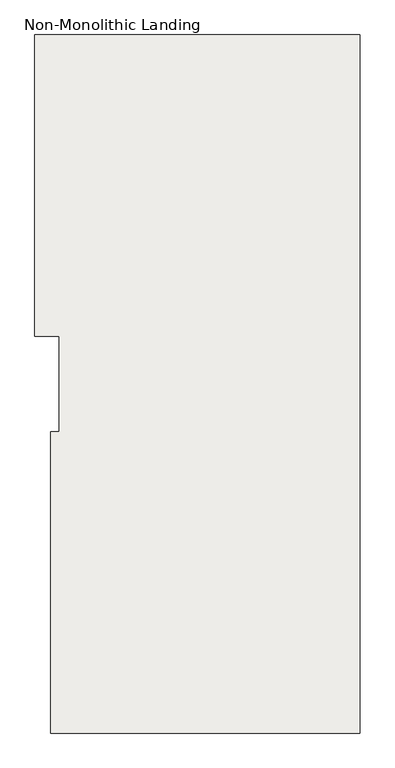
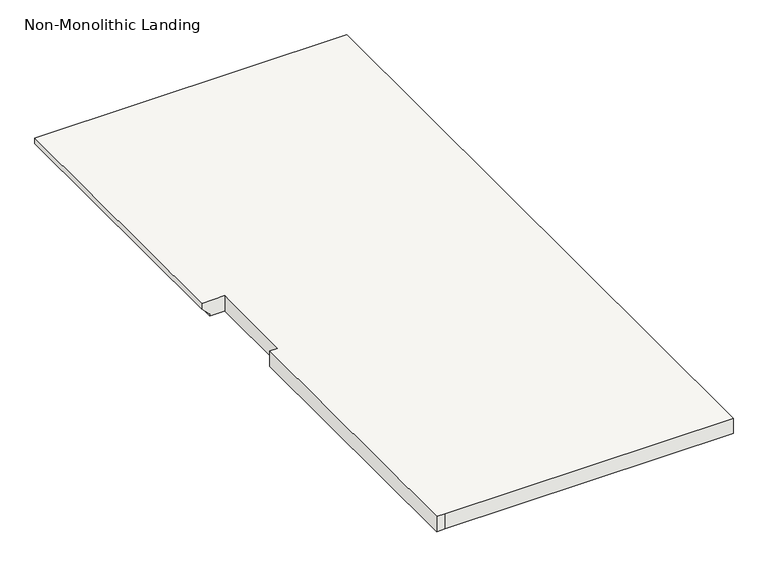
"""IFC4 building model written with IfcOpenShell, lengths in millimetres: slab geometry, Non-Monolithic Landing."""

from ifc_helpers import new_model, si_unit, origin, place, context, project, spatial, faceted_brep, source, transform, mapped, element, save


def non_monolithic_landing_a5fdca2b(model_context):
    return source(origin(), model_context, "Body", "Brep", [
        faceted_brep([(-6915.3703437, -6347.7504041, 4891.6166667), (-6915.3703437, -6347.7504041, 4910.6666667), (-6915.3703437, -5433.3504041, 4910.6666667), (-6915.3703437, -5433.3504041, 4891.6166667), (-6889.9703437, -6347.7504041, 4866.2166667), (-6889.9703437, -5433.3504041, 4866.2166667), (-6841.3260609, -6347.7504041, 4910.6666667), (-6841.3260609, -6639.0810793, 4910.6666667), (-6866.7260609, -6639.0810793, 4910.6666667), (-6866.7260609, -7553.4810793, 4910.6666667), (-6841.3260609, -7553.4810793, 4910.6666667), (-5926.9260609, -7553.4810793, 4910.6666667), (-5926.9260609, -5433.3504041, 4910.6666667), (-6889.9703437, -6347.7504041, 4859.8666667), (-6889.9703437, -5433.3504041, 4859.8666667), (-5926.9260609, -5433.3504041, 4859.8666667), (-5926.9260609, -7553.4810793, 4859.8666667), (-6841.3260609, -7553.4810793, 4859.8666667), (-6866.7260609, -7553.4810793, 4859.8666667), (-6866.7260609, -6639.0810793, 4859.8666667), (-6841.3260609, -6639.0810793, 4859.8666667), (-6841.3260609, -6347.7504041, 4859.8666667)], [[[0, 1, 2, 3]], [[4, 0, 3, 5]], [[6, 7, 8, 9, 10, 11, 12, 2, 1]], [[13, 14, 15, 16, 17, 18, 19, 20, 21]], [[14, 13, 4, 5]], [[6, 1, 0, 4, 13, 21]], [[7, 6, 21, 20]], [[8, 7, 20, 19]], [[9, 8, 19, 18]], [[10, 9, 18, 17]], [[11, 10, 17, 16]], [[12, 11, 16, 15]], [[2, 12, 15, 14, 5, 3]]]),
    ])


if __name__ == "__main__":
    model = new_model("IFC4")
    model_context = context("Model", 3, world=origin())
    ifc_project = project(units=[si_unit("LENGTHUNIT", "METRE", prefix="MILLI")], contexts=[model_context])
    site = spatial("IfcSite", under=ifc_project)
    building = spatial("IfcBuilding", under=site)
    placement = place(None, origin())
    non_monolithic_landing_shape = non_monolithic_landing_a5fdca2b(model_context)
    element("IfcSlab", 1, ObjectType="Non-Monolithic Landing", at=placement, inside=building, context=model_context, shape_type="MappedRepresentation", body=[
        mapped(non_monolithic_landing_shape, transform((0.0, 0.0, 0.0), x_axis=(1.0, 0.0, 0.0), y_axis=(0.0, 1.0, 0.0), z_axis=(0.0, 0.0, 1.0))),
    ])
    save(model, "model.ifc")
